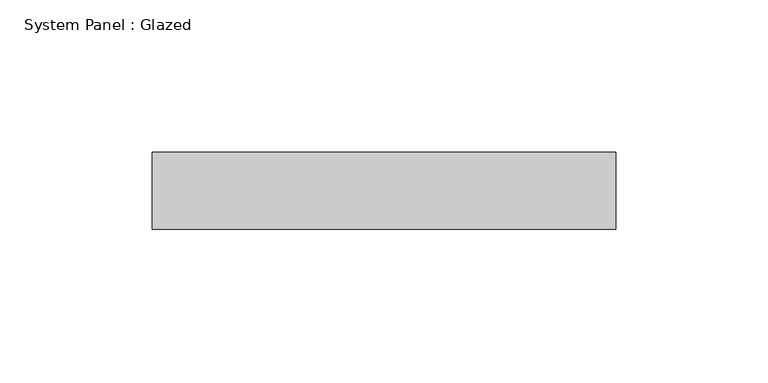
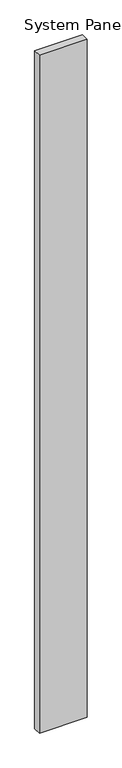
"""IFC4 building model written with IfcOpenShell, lengths in millimetres: plate geometry, System Panel : Glazed."""

from ifc_helpers import new_model, si_unit, origin, origin_with_axes, place, context, project, spatial, polyline, outline, extrude, source, transform, mapped, element, save


def system_panel_glazed_24bd3515(model_context):
    return source(origin(), model_context, "Body", "SweptSolid", [
        extrude(outline(polyline([(76.2, 19.05), (-76.2, 19.05), (-76.2, 44.45), (76.2, 44.45), (76.2, 19.05)])), origin_with_axes(), (0.0, 0.0, 1.0), 2287.5875),
    ])


if __name__ == "__main__":
    model = new_model("IFC4")
    model_context = context("Model", 3, world=origin())
    ifc_project = project(units=[si_unit("LENGTHUNIT", "METRE", prefix="MILLI")], contexts=[model_context])
    site = spatial("IfcSite", under=ifc_project)
    building = spatial("IfcBuilding", under=site)
    placement = place(None, origin())
    system_panel_glazed_shape = system_panel_glazed_24bd3515(model_context)
    element("IfcPlate", 1, ObjectType="System Panel : Glazed", at=placement, inside=building, context=model_context, shape_type="MappedRepresentation", body=[
        mapped(system_panel_glazed_shape, transform((0.0, 0.0, 0.0), x_axis=(1.0, 0.0, 0.0), y_axis=(0.0, 1.0, 0.0), z_axis=(0.0, 0.0, 1.0))),
    ])
    save(model, "model.ifc")

# Revit data of these elements
# Type "System Panel : Glazed"
#   Construction Type Id = "GSP4R"
#   Analytic Construction = "1/8 in Pilkington single glazing"
#   Visual Light Transmittance = 0.9
#   Solar Heat Gain Coefficient = 0.86
#   Heat Transfer Coefficient (U) = 1.18115 BTU/(h·ft²·°F)
#   Define Thermal Properties by = 1
# Element 1 (IfcPlate, "System Panel : Glazed")
#   Materials on its faces: "Glass"
# Materials
#   "Glass": class "Glass", colour RGB 0 128 192, transparency 0.75, Description = "Soda Lime Glass", Cost = 0
